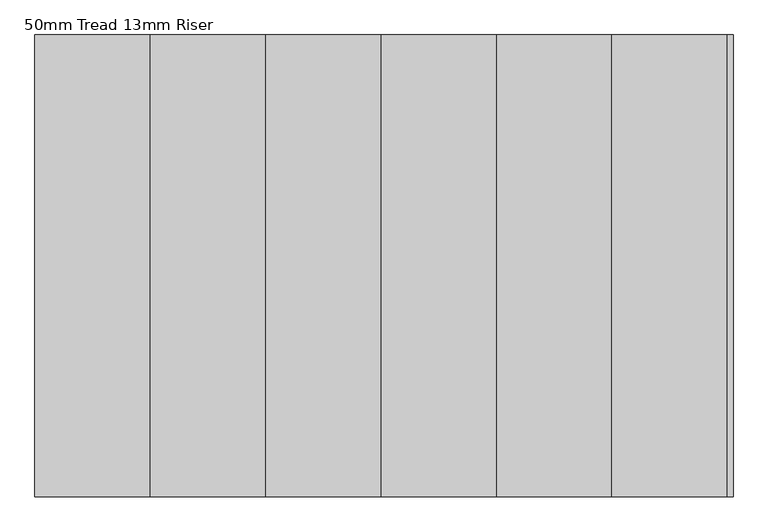
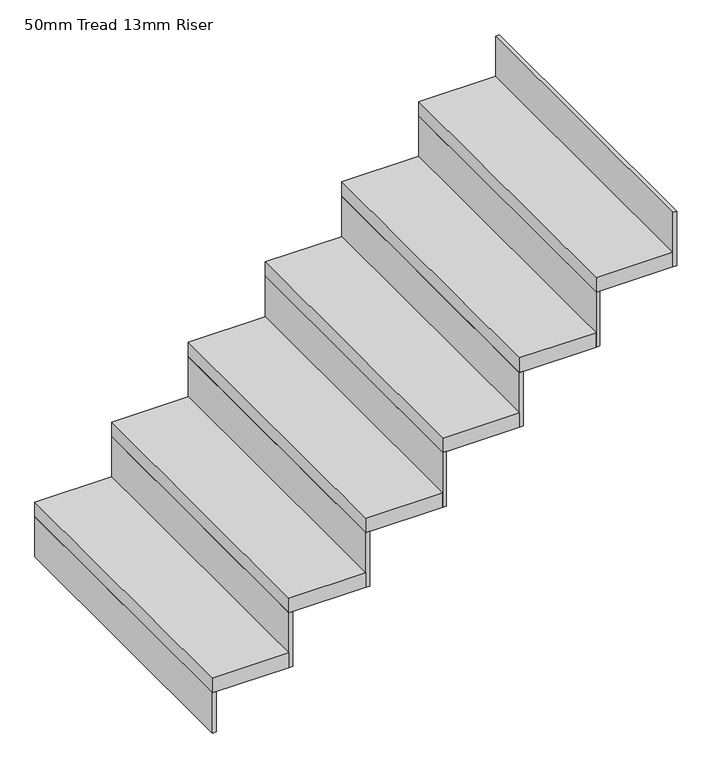
"""IFC4 building model written with IfcOpenShell, lengths in millimetres: stair flight geometry, 50mm Tread 13mm Riser."""

from ifc_helpers import new_model, si_unit, frame, origin, place, context, project, spatial, polyline, outline, extrude, source, transform, mapped, element, save


def stair_flight_50mm_tread_13mm_riser_c1773281(model_context):
    return source(origin(), model_context, "Body", "SweptSolid", [
        extrude(outline(polyline([(-11979.6794909, -2507.9876321), (-11992.1794909, -2507.9876321), (-11992.1794909, -1507.9618509), (-11979.6794909, -1507.9618509), (-11979.6794909, -2507.9876321)])), frame((0.0, 0.0, 6400.8), z_axis=(0.0, 0.0, 1.0), x_axis=(1.0, 0.0, 0.0)), (0.0, 0.0, 1.0), 138.2588235),
        extrude(outline(polyline([(-11742.1794909, -1507.9618509), (-11742.1794909, -2507.9876321), (-11992.1794909, -2507.9876321), (-11992.1794909, -1507.9618509), (-11742.1794909, -1507.9618509)])), frame((0.0, 0.0, 6539.0588235), z_axis=(0.0, 0.0, 1.0), x_axis=(1.0, 0.0, 0.0)), (0.0, 0.0, 1.0), 50.0),
        extrude(outline(polyline([(-11729.6794909, -2507.9876321), (-11742.1794909, -2507.9876321), (-11742.1794909, -1507.9618509), (-11729.6794909, -1507.9618509), (-11729.6794909, -2507.9876321)])), frame((0.0, 0.0, 6539.0588235), z_axis=(0.0, 0.0, 1.0), x_axis=(1.0, 0.0, 0.0)), (0.0, 0.0, 1.0), 188.2588235),
        extrude(outline(polyline([(-11492.1794909, -1507.9618509), (-11492.1794909, -2507.9876321), (-11742.1794909, -2507.9876321), (-11742.1794909, -1507.9618509), (-11492.1794909, -1507.9618509)])), frame((0.0, 0.0, 6727.3176471), z_axis=(0.0, 0.0, 1.0), x_axis=(1.0, 0.0, 0.0)), (0.0, 0.0, 1.0), 50.0),
        extrude(outline(polyline([(-11479.6794909, -2507.9876321), (-11492.1794909, -2507.9876321), (-11492.1794909, -1507.9618509), (-11479.6794909, -1507.9618509), (-11479.6794909, -2507.9876321)])), frame((0.0, 0.0, 6727.3176471), z_axis=(0.0, 0.0, 1.0), x_axis=(1.0, 0.0, 0.0)), (0.0, 0.0, 1.0), 188.2588235),
        extrude(outline(polyline([(-11242.1794909, -1507.9618509), (-11242.1794909, -2507.9876321), (-11492.1794909, -2507.9876321), (-11492.1794909, -1507.9618509), (-11242.1794909, -1507.9618509)])), frame((0.0, 0.0, 6915.5764706), z_axis=(0.0, 0.0, 1.0), x_axis=(1.0, 0.0, 0.0)), (0.0, 0.0, 1.0), 50.0),
        extrude(outline(polyline([(-11229.6794909, -2507.9876321), (-11242.1794909, -2507.9876321), (-11242.1794909, -1507.9618509), (-11229.6794909, -1507.9618509), (-11229.6794909, -2507.9876321)])), frame((0.0, 0.0, 6915.5764706), z_axis=(0.0, 0.0, 1.0), x_axis=(1.0, 0.0, 0.0)), (0.0, 0.0, 1.0), 188.2588235),
        extrude(outline(polyline([(-10992.1794909, -1507.9618509), (-10992.1794909, -2507.9876321), (-11242.1794909, -2507.9876321), (-11242.1794909, -1507.9618509), (-10992.1794909, -1507.9618509)])), frame((0.0, 0.0, 7103.8352941), z_axis=(0.0, 0.0, 1.0), x_axis=(1.0, 0.0, 0.0)), (0.0, 0.0, 1.0), 50.0),
        extrude(outline(polyline([(-10979.6794909, -2507.9876321), (-10992.1794909, -2507.9876321), (-10992.1794909, -1507.9618509), (-10979.6794909, -1507.9618509), (-10979.6794909, -2507.9876321)])), frame((0.0, 0.0, 7103.8352941), z_axis=(0.0, 0.0, 1.0), x_axis=(1.0, 0.0, 0.0)), (0.0, 0.0, 1.0), 188.2588235),
        extrude(outline(polyline([(-10742.1794909, -1507.9618509), (-10742.1794909, -2507.9876321), (-10992.1794909, -2507.9876321), (-10992.1794909, -1507.9618509), (-10742.1794909, -1507.9618509)])), frame((0.0, 0.0, 7292.0941176), z_axis=(0.0, 0.0, 1.0), x_axis=(1.0, 0.0, 0.0)), (0.0, 0.0, 1.0), 50.0),
        extrude(outline(polyline([(-10729.6794909, -2507.9876321), (-10742.1794909, -2507.9876321), (-10742.1794909, -1507.9618509), (-10729.6794909, -1507.9618509), (-10729.6794909, -2507.9876321)])), frame((0.0, 0.0, 7292.0941176), z_axis=(0.0, 0.0, 1.0), x_axis=(1.0, 0.0, 0.0)), (0.0, 0.0, 1.0), 188.2588235),
        extrude(outline(polyline([(-10479.6794909, -2507.9876321), (-10492.1794909, -2507.9876321), (-10492.1794909, -1507.9618509), (-10479.6794909, -1507.9618509), (-10479.6794909, -2507.9876321)])), frame((0.0, 0.0, 7480.3529412), z_axis=(0.0, 0.0, 1.0), x_axis=(1.0, 0.0, 0.0)), (0.0, 0.0, 1.0), 188.2588235),
        extrude(outline(polyline([(-10492.1794909, -1507.9618509), (-10492.1794909, -2507.9876321), (-10742.1794909, -2507.9876321), (-10742.1794909, -1507.9618509), (-10492.1794909, -1507.9618509)])), frame((0.0, 0.0, 7480.3529412), z_axis=(0.0, 0.0, 1.0), x_axis=(1.0, 0.0, 0.0)), (0.0, 0.0, 1.0), 50.0),
    ])


if __name__ == "__main__":
    model = new_model("IFC4")
    model_context = context("Model", 3, world=origin())
    ifc_project = project(units=[si_unit("LENGTHUNIT", "METRE", prefix="MILLI")], contexts=[model_context])
    site = spatial("IfcSite", under=ifc_project)
    building = spatial("IfcBuilding", under=site)
    placement = place(None, origin())
    stair_flight_50mm_tread_13mm_riser_shape = stair_flight_50mm_tread_13mm_riser_c1773281(model_context)
    element("IfcStairFlight", 1, ObjectType="50mm Tread 13mm Riser", at=placement, inside=building, context=model_context, shape_type="MappedRepresentation", body=[
        mapped(stair_flight_50mm_tread_13mm_riser_shape, transform((0.0, 0.0, 0.0), x_axis=(1.0, 0.0, 0.0), y_axis=(0.0, 1.0, 0.0), z_axis=(0.0, 0.0, 1.0))),
    ])
    save(model, "model.ifc")
